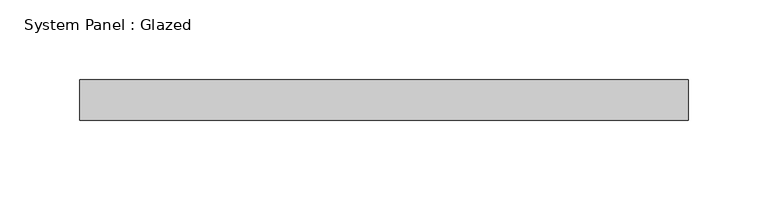
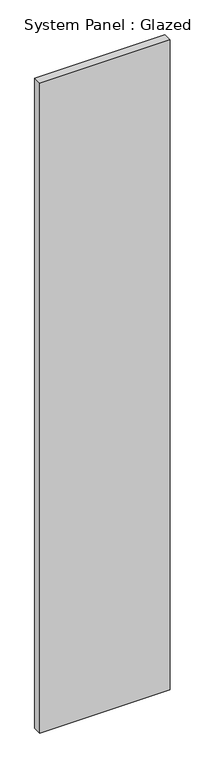
"""IFC4 building model written with IfcOpenShell, lengths in millimetres: plate geometry, System Panel : Glazed."""

from ifc_helpers import new_model, si_unit, origin, origin_with_axes, place, context, project, spatial, polyline, outline, extrude, source, transform, mapped, element, save


def system_panel_glazed_dc74cd20(model_context):
    return source(origin(), model_context, "Body", "SweptSolid", [
        extrude(outline(polyline([(190.5, 19.05), (-190.5, 19.05), (-190.5, 44.45), (190.5, 44.45), (190.5, 19.05)])), origin_with_axes(), (0.0, 0.0, 1.0), 2006.6),
    ])


if __name__ == "__main__":
    model = new_model("IFC4")
    model_context = context("Model", 3, world=origin())
    ifc_project = project(units=[si_unit("LENGTHUNIT", "METRE", prefix="MILLI")], contexts=[model_context])
    site = spatial("IfcSite", under=ifc_project)
    building = spatial("IfcBuilding", under=site)
    placement = place(None, origin())
    system_panel_glazed_shape = system_panel_glazed_dc74cd20(model_context)
    element("IfcPlate", 1, ObjectType="System Panel : Glazed", at=placement, inside=building, context=model_context, shape_type="MappedRepresentation", body=[
        mapped(system_panel_glazed_shape, transform((0.0, 0.0, 0.0), x_axis=(1.0, 0.0, 0.0), y_axis=(0.0, 1.0, 0.0), z_axis=(0.0, 0.0, 1.0))),
    ])
    save(model, "model.ifc")

# Revit data of these elements
# Type "System Panel : Glazed"
#   Construction Type Id = "GSP4R"
#   Analytic Construction = "1/8 in Pilkington single glazing"
#   Visual Light Transmittance = 0.9
#   Solar Heat Gain Coefficient = 0.86
#   Heat Transfer Coefficient (U) = 1.18115 BTU/(h·ft²·°F)
#   Define Thermal Properties by = 1
# Element 1 (IfcPlate, "System Panel : Glazed")
#   Materials on its faces: "Glass"
# Materials
#   "Glass": class "Glass", colour RGB 0 128 192, transparency 0.75, Description = "Soda Lime Glass", Cost = 0
